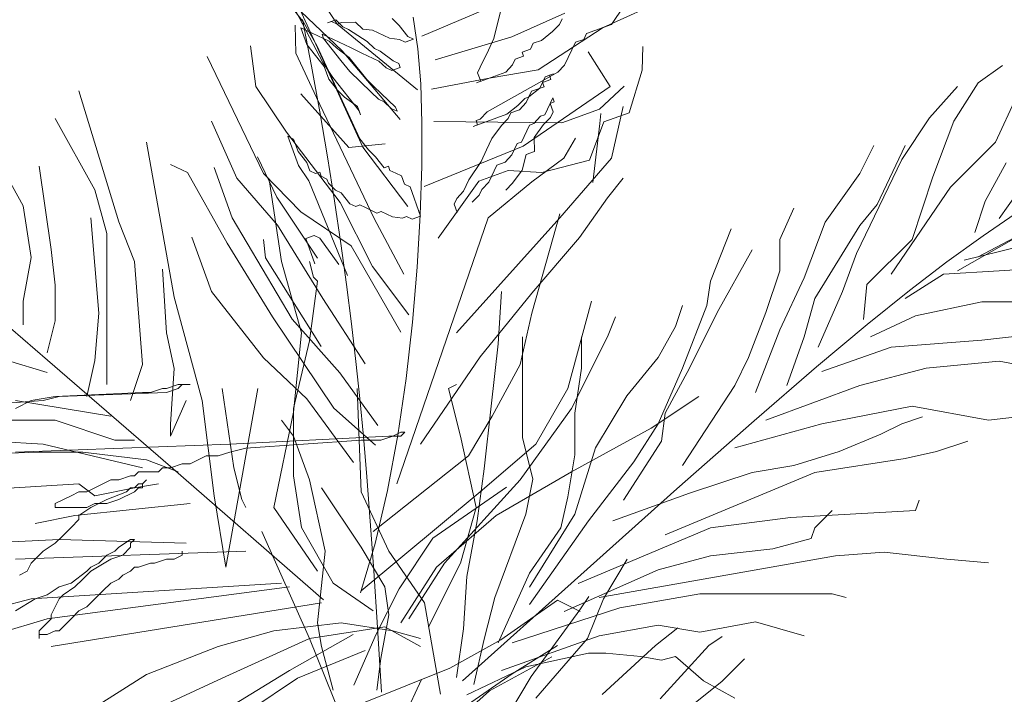
# Model space of a CAD drawing. Units: millimetres. Extents: x 595116 to 630915, y 909473 to 920225.
# Tile 37 of 134: x 629665.643 to 629671.98, y 919173.119 to 919177.461. Entities that reach past the tile are written whole.
import ezdxf

# ---------------------------------------------------------------- set-up
doc = ezdxf.new("R2010")
doc.units = ezdxf.units.MM
doc.layers.add('Dimension', color=3, linetype='Continuous', lineweight=18)
doc.layers.add('L-PLNT', color=85, linetype='Continuous', lineweight=13)
doc.styles.get("Standard").update_dxf_attribs({"font": 'arial.ttf'})
doc.dimstyles.new('ISO-25', dxfattribs={"dimtxt": 9, "dimasz": 6, "dimexe": 1.25, "dimexo": 0.625, "dimtad": 1, "dimlunit": 4, "dimtxsty": 'Standard', "dimcen": 2.5, "dimadec": 0, "dimazin": 0, "dimtfac": 1, "dimtmove": 0, "dimatfit": 3, "dimfxl": 1, "dimarcsym": 0})

# ---------------------------------------------------------------- blocks, each defined once
blk = doc.blocks.new('A$C4FB75ABC')
for p, q in [((2.6801, 3.4593), (2.5376, 3.6754)), ((2.6552, 3.3935), (2.5769, 3.5437)), ((3.136, 3.4531), (3.303, 3.5294)), ((2.6885, 3.4136), (2.5774, 3.5196)), ((2.5924, 3.5006), (2.6222, 3.4627)), ((2.7237, 3.248), (2.6067, 3.5058)), ((2.8253, 3.4385), (2.9518, 3.4922)), ((2.9484, 3.4342), (2.9616, 3.4876)), ((2.9797, 3.4374), (3.0703, 3.4781)), ((3.1503, 3.4583), (3.1713, 3.4901)), ((2.636, 3.3873), (2.6204, 3.467)), ((2.6222, 3.4627), (2.6449, 3.4222)), ((2.6632, 3.4613), (2.6776, 3.4664)), ((2.6704, 3.4639), (2.6632, 3.4613)), ((2.6801, 3.4593), (2.6704, 3.4639)), ((2.6776, 3.4664), (2.6899, 3.4547)), ((2.6873, 3.4618), (2.6801, 3.4593)), ((2.7114, 3.4624), (2.6873, 3.4618)), ((2.7237, 3.4506), (2.7114, 3.4624)), ((2.774, 3.4687), (2.7863, 3.4569)), ((2.81, 3.4712), (2.8183, 3.4166)), ((3.0657, 3.4683), (3.0611, 3.4586)), ((2.609, 3.4093), (2.6078, 3.4576)), ((2.6566, 3.4346), (2.6176, 3.453)), ((2.6176, 3.453), (2.6279, 3.4243)), ((2.8178, 3.3467), (2.6801, 3.4593)), ((2.6899, 3.4547), (2.6996, 3.4501)), ((2.6996, 3.4501), (2.7315, 3.4291)), ((2.7407, 3.4486), (2.7237, 3.4506)), ((2.7699, 3.4348), (2.7407, 3.4486)), ((2.7863, 3.4569), (2.8012, 3.438)), ((3.0244, 3.3805), (3.136, 3.4531)), ((3.0494, 3.4462), (3.0304, 3.4313)), ((3.0611, 3.4586), (3.0494, 3.4462)), ((3.1073, 3.4428), (3.1503, 3.4583)), ((2.6638, 3.4372), (2.654, 3.4418)), ((2.654, 3.4418), (2.6566, 3.4346)), ((2.6566, 3.4346), (2.6664, 3.43)), ((2.6865, 3.3967), (2.6566, 3.4346)), ((2.693, 3.4234), (2.6638, 3.4372)), ((2.6664, 3.43), (2.6787, 3.4182)), ((2.7315, 3.4291), (2.7438, 3.4173)), ((2.7869, 3.4328), (2.7699, 3.4348)), ((2.7966, 3.4282), (2.7869, 3.4328)), ((2.811, 3.4334), (2.7966, 3.4282)), ((2.8012, 3.438), (2.811, 3.4334)), ((2.848, 3.3981), (2.9797, 3.4374)), ((2.9392, 3.4147), (2.9484, 3.4342)), ((3.0304, 3.4313), (3.0161, 3.4262)), ((3.07, 3.3888), (3.0884, 3.4279)), ((3.0884, 3.4279), (3.1027, 3.433)), ((3.1027, 3.433), (3.1073, 3.4428)), ((2.5404, 3.3522), (2.5315, 3.422)), ((2.6279, 3.4243), (2.6578, 3.3864)), ((2.6449, 3.4222), (2.7186, 3.2624)), ((2.6787, 3.4182), (2.7008, 3.4019)), ((2.7877, 3.2953), (2.6885, 3.4136)), ((2.7028, 3.4188), (2.693, 3.4234)), ((2.7223, 3.4096), (2.7028, 3.4188)), ((2.7438, 3.4173), (2.7536, 3.4127)), ((2.7536, 3.4127), (2.7757, 3.3964)), ((2.8183, 3.4166), (2.8233, 3.3565)), ((2.9254, 3.3854), (2.9392, 3.4147)), ((3.0115, 3.4164), (2.9972, 3.4112)), ((2.9972, 3.4112), (2.9997, 3.4041)), ((3.0161, 3.4262), (3.0115, 3.4164)), ((3.1481, 3.3521), (3.1105, 3.4115)), ((3.2028, 3.3799), (3.2043, 3.4209)), ((2.5536, 3.203), (2.4572, 3.4034)), ((2.6446, 3.333), (2.609, 3.4093)), ((2.6727, 3.3674), (2.6552, 3.3935)), ((2.7014, 3.3777), (2.6865, 3.3967)), ((2.7008, 3.4019), (2.7306, 3.364)), ((2.7516, 3.3958), (2.7223, 3.4096)), ((2.7639, 3.384), (2.7516, 3.3958)), ((2.7757, 3.3964), (2.7854, 3.3918)), ((2.9854, 3.3989), (2.9808, 3.3891)), ((2.9997, 3.4041), (2.9854, 3.3989)), ((2.6503, 3.3086), (2.636, 3.3873)), ((2.6578, 3.3864), (2.6655, 3.3648)), ((2.7384, 3.3424), (2.7014, 3.3777)), ((2.7737, 3.3794), (2.7639, 3.384)), ((2.788, 3.3846), (2.7737, 3.3794)), ((2.7854, 3.3918), (2.788, 3.3846)), ((2.969, 3.3768), (2.9188, 3.3587)), ((2.9208, 3.3757), (2.9254, 3.3854)), ((2.9369, 3.3085), (3.0583, 3.3765)), ((2.9403, 3.3665), (3.0244, 3.3805)), ((2.9808, 3.3891), (2.969, 3.3768)), ((3.0583, 3.3765), (3.07, 3.3888)), ((3.1805, 3.307), (3.2028, 3.3799)), ((3.7791, 3.3582), (3.8208, 3.388)), ((2.6655, 3.3648), (2.6804, 3.3459)), ((2.7174, 3.3106), (2.6727, 3.3674)), ((2.7306, 3.364), (2.743, 3.3522)), ((2.8419, 3.3473), (2.9403, 3.3665)), ((2.9188, 3.3587), (2.926, 3.3613)), ((2.926, 3.3613), (2.9208, 3.3757)), ((3.0367, 3.3687), (3.0322, 3.359)), ((3.0322, 3.359), (3.0465, 3.3642)), ((3.0511, 3.3739), (3.0367, 3.3687)), ((3.0439, 3.3713), (3.0511, 3.3739)), ((3.0465, 3.3642), (3.0439, 3.3713)), ((2.2372, 3.345), (2.3054, 3.1203)), ((2.5929, 3.2739), (2.5404, 3.3522)), ((2.6804, 3.3459), (2.6928, 3.3341)), ((2.743, 3.3522), (2.7553, 3.3404)), ((2.8233, 3.3565), (2.8254, 3.2898)), ((2.9986, 3.2497), (3.1481, 3.3521)), ((3.0276, 3.3492), (3.0086, 3.3343)), ((3.0086, 3.3343), (3.0132, 3.3441)), ((3.0132, 3.3441), (3.0347, 3.3518)), ((3.0322, 3.359), (3.0276, 3.3492)), ((3.0347, 3.3518), (3.0322, 3.359)), ((3.1297, 3.313), (3.1722, 3.3526)), ((3.6956, 3.2986), (3.7433, 3.3522)), ((3.7373, 3.2926), (3.7791, 3.3582)), ((2.6997, 3.2474), (2.6179, 3.3396)), ((2.7435, 3.1255), (2.6446, 3.333)), ((2.6928, 3.3341), (2.7149, 3.3178)), ((2.7507, 3.3307), (2.7384, 3.3424)), ((2.7605, 3.3261), (2.7507, 3.3307)), ((2.7553, 3.3404), (2.78, 3.3169)), ((2.7728, 3.3143), (2.7605, 3.3261)), ((3.0015, 3.3317), (2.9897, 3.3194)), ((3.0086, 3.3343), (3.0015, 3.3317)), ((3.004, 3.3246), (3.0086, 3.3343)), ((3.0497, 3.3329), (3.0451, 3.3231)), ((3.0522, 3.3257), (3.0497, 3.3329)), ((3.8089, 3.2568), (3.8447, 3.3343)), ((2.7149, 3.3178), (2.72, 3.3034)), ((2.72, 3.3034), (2.7174, 3.3106)), ((2.7826, 3.3097), (2.7728, 3.3143)), ((2.78, 3.3169), (2.7826, 3.3097)), ((2.9897, 3.3194), (2.9708, 3.3045)), ((2.9779, 3.3071), (2.9923, 3.3122)), ((2.9923, 3.3122), (3.004, 3.3246)), ((3.0359, 3.3036), (3.0405, 3.3134)), ((3.0405, 3.3134), (3.0451, 3.3231)), ((3.0451, 3.3231), (3.0522, 3.3257)), ((3.0451, 3.3231), (3.0502, 3.3088)), ((3.0651, 3.2898), (3.1297, 3.313)), ((3.1501, 3.2292), (3.1706, 3.3178)), ((2.1963, 3.2973), (2.2645, 3.1748)), ((2.508, 3.1947), (2.4647, 3.2926)), ((2.6635, 3.2315), (2.6503, 3.3086)), ((2.9708, 3.3045), (2.9134, 3.2838)), ((2.918, 3.2936), (2.9251, 3.2962)), ((2.9206, 3.2864), (2.918, 3.2936)), ((2.9251, 3.2962), (2.9369, 3.3085)), ((2.9616, 3.285), (2.9733, 3.2973)), ((2.9733, 3.2973), (2.9779, 3.3071)), ((3.0169, 3.2887), (3.0287, 3.301)), ((3.0287, 3.301), (3.0359, 3.3036)), ((3.0456, 3.299), (3.0339, 3.2867)), ((3.0502, 3.3088), (3.0456, 3.299)), ((3.1303, 3.2889), (3.1323, 3.3059)), ((3.1374, 3.2915), (3.1805, 3.307)), ((3.6479, 3.227), (3.6956, 3.2986)), ((3.7015, 3.1972), (3.7373, 3.2926)), ((2.8254, 3.2898), (2.825, 3.2153)), ((2.8457, 3.2919), (3.0651, 3.2898)), ((2.9134, 3.2838), (2.9206, 3.2864)), ((2.9452, 3.2629), (2.9616, 3.285)), ((2.996, 3.2568), (3.0052, 3.2763)), ((3.0052, 3.2763), (3.0098, 3.2861)), ((3.0098, 3.2861), (3.0169, 3.2887)), ((3.0339, 3.2867), (3.0175, 3.2646)), ((3.1125, 3.2258), (3.1374, 3.2915)), ((3.1182, 3.1873), (3.1303, 3.2889)), ((2.685, 3.153), (2.5929, 3.2739)), ((2.6053, 3.2621), (2.5955, 3.2667)), ((2.5955, 3.2667), (2.6136, 3.2165)), ((2.613, 3.2406), (2.6053, 3.2621)), ((2.7186, 3.2624), (2.7335, 3.2434)), ((2.936, 3.2434), (2.9452, 3.2629)), ((3.0175, 3.2646), (3.0181, 3.2405)), ((3.0684, 3.2292), (3.0888, 3.2633)), ((2.353, 3.2565), (2.4007, 2.9909)), ((2.7622, 3.2537), (2.6997, 3.2474)), ((2.8009, 3.1461), (2.7237, 3.248)), ((2.7335, 3.2434), (2.7458, 3.2316)), ((2.829, 3.1805), (2.9986, 3.2497)), ((2.9269, 3.2238), (2.936, 3.2434)), ((2.9797, 3.2347), (2.9842, 3.2445)), ((2.9842, 3.2445), (2.9888, 3.2542)), ((2.9888, 3.2542), (2.996, 3.2568)), ((3.5763, 3.2032), (3.6001, 3.2509)), ((3.6061, 3.1495), (3.6538, 3.2509)), ((3.7314, 3.1793), (3.8089, 3.2568)), ((2.5763, 3.1625), (2.5433, 3.2317)), ((2.6279, 3.2216), (2.613, 3.2406)), ((2.6754, 3.1561), (2.6635, 3.2315)), ((2.7458, 3.2316), (2.7608, 3.2127)), ((2.9679, 3.2224), (2.9797, 3.2347)), ((3.0038, 3.2353), (2.9972, 3.2086)), ((3.0181, 3.2405), (3.0038, 3.2353)), ((3.0139, 3.1884), (3.0684, 3.2292)), ((3.031, 3.2046), (3.1125, 3.2258)), ((3.0616, 3.1271), (3.1501, 3.2292)), ((3.5703, 3.066), (3.6479, 3.227)), ((3.8149, 3.1257), (3.8865, 3.227)), ((2.1078, 3.2088), (2.1418, 3.1475)), ((2.1691, 3.2156), (2.1895, 3.0726)), ((2.4234, 3.2048), (2.3941, 3.2186)), ((2.5, 3.127), (2.469, 3.2131)), ((2.6136, 3.2165), (2.6311, 3.1904)), ((2.6331, 3.2073), (2.6279, 3.2216)), ((2.7608, 3.2127), (2.7679, 3.2153)), ((2.7679, 3.2153), (2.7705, 3.2081)), ((2.7705, 3.2081), (2.7803, 3.2035)), ((2.825, 3.2153), (2.8223, 3.1323)), ((2.9059, 3.192), (2.9269, 3.2238)), ((2.9229, 3.19), (2.9731, 3.208)), ((2.949, 3.2075), (2.9535, 3.2172)), ((2.9535, 3.2172), (2.9679, 3.2224)), ((2.9731, 3.208), (3.031, 3.2046)), ((2.9972, 3.2086), (2.9808, 3.1865)), ((3.791, 3.1555), (3.8268, 3.2211)), ((2.4914, 3.0833), (2.4234, 3.2048)), ((2.5774, 3.1143), (2.508, 3.1947)), ((2.6179, 3.137), (2.5536, 3.203)), ((2.6428, 3.2027), (2.6331, 3.2073)), ((2.65, 3.2053), (2.6428, 3.2027)), ((2.6526, 3.1981), (2.65, 3.2053)), ((2.6624, 3.1935), (2.6526, 3.1981)), ((2.6649, 3.1863), (2.6624, 3.1935)), ((2.7803, 3.2035), (2.79, 3.1989)), ((2.79, 3.1989), (2.7952, 3.1846)), ((2.8967, 3.1725), (2.9059, 3.192)), ((2.9398, 3.188), (2.949, 3.2075)), ((3.1433, 3.1611), (3.1706, 3.1952)), ((3.5166, 3.1197), (3.5763, 3.2032)), ((3.6658, 3.0899), (3.7015, 3.1972)), ((2.2645, 3.1748), (2.2849, 3.0999)), ((2.5847, 3.0522), (2.5642, 3.1884)), ((2.6311, 3.1904), (2.6976, 3.0279)), ((2.6773, 3.1746), (2.6649, 3.1863)), ((2.687, 3.17), (2.6773, 3.1746)), ((2.7952, 3.1846), (2.8049, 3.18)), ((2.8049, 3.18), (2.823, 3.1297)), ((2.8529, 3.0918), (2.9229, 3.19)), ((2.9234, 3.1659), (2.928, 3.1756)), ((2.928, 3.1756), (2.9398, 3.188)), ((2.9389, 3.1271), (3.0139, 3.1884)), ((2.9808, 3.1865), (2.969, 3.1742)), ((3.63, 3.0303), (3.7314, 3.1793)), ((2.6463, 3.058), (2.5763, 3.1625)), ((2.7019, 3.151), (2.687, 3.17)), ((2.8804, 3.1504), (2.885, 3.1601)), ((2.885, 3.1601), (2.8967, 3.1725)), ((2.9117, 3.1535), (2.9234, 3.1659)), ((3.0956, 3.093), (3.1433, 3.1611)), ((2.1418, 3.1475), (2.1555, 3.059)), ((2.6863, 3.0831), (2.6754, 3.1561)), ((2.7407, 3.0434), (2.685, 3.153)), ((2.7117, 3.1464), (2.7019, 3.151)), ((2.7189, 3.149), (2.7117, 3.1464)), ((2.7286, 3.1444), (2.7189, 3.149)), ((2.7481, 3.1352), (2.7286, 3.1444)), ((2.8856, 3.136), (2.8804, 3.1504)), ((3.4391, 3.0899), (3.4629, 3.1436)), ((3.5763, 3.1137), (3.6061, 3.1495)), ((3.7731, 3.1018), (3.791, 3.1555)), ((2.2577, 3.1271), (2.2713, 2.9637)), ((2.603, 2.9533), (2.5, 3.127)), ((2.7037, 3.0787), (2.6179, 3.137)), ((2.794, 3.0302), (2.7435, 3.1255)), ((2.7553, 3.1378), (2.7481, 3.1352)), ((2.7651, 3.1332), (2.7553, 3.1378)), ((2.7748, 3.1286), (2.7651, 3.1332)), ((2.7917, 3.1266), (2.7748, 3.1286)), ((2.7823, 2.6709), (2.9389, 3.1271)), ((2.7989, 3.1292), (2.7917, 3.1266)), ((2.8087, 3.1246), (2.7989, 3.1292)), ((2.823, 3.1297), (2.8087, 3.1246)), ((2.8223, 3.1323), (2.817, 3.0425)), ((2.8844, 2.9296), (3.0616, 3.1271)), ((3.0139, 2.9637), (3.0616, 3.1339)), ((3.7873, 3.0958), (3.8516, 3.1401)), ((2.3054, 3.1203), (2.3326, 3.0522)), ((2.6552, 2.9883), (2.5774, 3.1143)), ((3.3198, 3.0184), (3.3556, 3.1078)), ((3.4808, 3.0243), (3.5166, 3.1197)), ((3.4987, 2.9885), (3.5763, 3.1137)), ((3.7433, 3.0362), (3.8805, 3.1137)), ((3.7791, 3.0601), (3.8805, 3.1137)), ((2.2849, 3.0999), (2.2849, 2.9024)), ((2.4644, 3.0007), (2.4308, 3.094)), ((2.5571, 3.0584), (2.5539, 3.0896)), ((2.6406, 3.0965), (2.6262, 3.0913)), ((2.6262, 3.0913), (2.6417, 3.0483)), ((2.6503, 3.0919), (2.6406, 3.0965)), ((2.6827, 3.0468), (2.6503, 3.0919)), ((3.0139, 2.9977), (3.0956, 3.093)), ((3.4391, 3.0362), (3.4391, 3.0899)), ((3.5882, 3.0124), (3.6658, 3.0899)), ((3.7254, 3.0513), (3.7873, 3.0958)), ((2.1895, 3.0726), (2.1963, 3.0113)), ((2.5691, 2.9573), (2.4914, 3.0833)), ((2.696, 3.0126), (2.6863, 3.0831)), ((2.7892, 2.9311), (2.7037, 3.0787)), ((3.7552, 3.0541), (3.8507, 3.078)), ((2.1555, 3.059), (2.1418, 2.9841)), ((2.6523, 2.9062), (2.5571, 3.0584)), ((3.3317, 2.9647), (3.3914, 3.072)), ((3.5465, 3.0005), (3.5703, 3.066)), ((2.3326, 3.0522), (2.3462, 2.8751)), ((2.6187, 2.9296), (2.5847, 3.0522)), ((2.6392, 3.0249), (2.6324, 3.0522)), ((2.8029, 2.9604), (2.7407, 3.0434)), ((2.817, 3.0425), (2.809, 2.948)), ((3.6611, 3.0024), (3.7254, 3.0513)), ((3.8149, 3.0362), (3.9222, 3.0422)), ((2.1835, 2.8826), (2.0174, 3.0255)), ((2.3803, 3.0386), (2.3871, 2.9296)), ((2.646, 3.0181), (2.6392, 3.0249)), ((3.4152, 2.9647), (3.4391, 3.0362)), ((3.4391, 2.9349), (3.4808, 3.0243)), ((3.6538, 2.9885), (3.7194, 3.0303)), ((3.7194, 3.0303), (3.8149, 3.0362)), ((2.1963, 3.0113), (2.1963, 2.95)), ((2.6324, 2.916), (2.646, 3.0181)), ((2.7046, 2.9452), (2.696, 3.0126)), ((3.3138, 2.9766), (3.3198, 3.0184)), ((3.5822, 2.9528), (3.5882, 3.0124)), ((2.4007, 2.9909), (2.4484, 2.8139)), ((2.5539, 2.887), (2.4644, 3.0007)), ((2.7278, 2.8766), (2.6552, 2.9883)), ((2.9253, 2.8888), (3.0139, 2.9977)), ((2.9559, 2.911), (2.9619, 3.0005)), ((3.4808, 2.923), (3.4987, 2.9885)), ((3.5047, 2.9051), (3.5465, 3.0005)), ((3.5886, 2.9442), (3.6611, 3.0024)), ((2.1418, 2.9841), (2.1418, 2.9432)), ((3.0752, 2.8343), (3.1161, 2.9841)), ((3.2601, 2.9408), (3.2721, 2.9766)), ((3.2721, 2.8693), (3.3138, 2.9766)), ((3.6717, 2.9587), (3.7851, 2.9826)), ((3.7851, 2.9826), (3.8745, 2.9826)), ((2.2713, 2.9637), (2.2645, 2.882)), ((2.6741, 2.8006), (2.5691, 2.9573)), ((2.9935, 2.8751), (3.0139, 2.9637)), ((3.1433, 2.9228), (3.157, 2.9569)), ((3.284, 2.8693), (3.3317, 2.9647)), ((3.3854, 2.8872), (3.4152, 2.9647)), ((3.5942, 2.923), (3.6717, 2.9587)), ((2.1963, 2.95), (2.1827, 2.8956)), ((2.6847, 2.8611), (2.603, 2.9533)), ((2.7122, 2.8807), (2.7046, 2.9452)), ((2.809, 2.948), (2.7981, 2.8512)), ((3.2303, 2.8872), (3.2601, 2.9408)), ((3.5019, 2.8714), (3.5886, 2.9442)), ((2.3871, 2.9296), (2.4007, 2.8683)), ((2.6051, 2.7934), (2.6187, 2.9296)), ((2.9977, 2.8216), (2.9977, 2.923)), ((3.082, 2.8002), (3.1433, 2.9228)), ((3.0991, 2.8693), (3.0991, 2.923)), ((3.3973, 2.8276), (3.4391, 2.9349)), ((3.451, 2.8395), (3.4808, 2.923)), ((3.7851, 2.917), (3.8924, 2.9289)), ((2.6051, 2.8002), (2.6324, 2.916)), ((2.944, 2.8037), (2.9559, 2.911)), ((3.5107, 2.8633), (3.63, 2.9051)), ((3.63, 2.9051), (3.7851, 2.917)), ((2.2849, 2.9024), (2.2849, 2.8411)), ((2.6279, 2.8164), (2.5539, 2.887)), ((2.8231, 2.739), (2.9253, 2.8888)), ((3.1766, 2.8216), (3.2303, 2.8872)), ((3.3615, 2.8395), (3.3854, 2.8872)), ((2.1146, 2.882), (2.1827, 2.8615)), ((2.3943, 2.7002), (2.1835, 2.8826)), ((2.2645, 2.882), (2.2508, 2.8207)), ((2.3462, 2.8751), (2.3258, 2.8139)), ((2.7189, 2.8171), (2.7122, 2.8807)), ((2.9458, 2.7866), (2.9935, 2.8751)), ((3.3951, 2.779), (3.5019, 2.8714)), ((3.6896, 2.8693), (3.8149, 2.8812)), ((3.8149, 2.8812), (3.9103, 2.8633)), ((2.4007, 2.8683), (2.3939, 2.773)), ((2.7496, 2.771), (2.6847, 2.8611)), ((3.0872, 2.7918), (3.0991, 2.8693)), ((3.2303, 2.7739), (3.2721, 2.8693)), ((3.2422, 2.7918), (3.284, 2.8693)), ((3.5763, 2.8395), (3.6896, 2.8693)), ((2.3871, 2.8343), (2.4075, 2.8411)), ((2.4075, 2.8411), (2.428, 2.8411)), ((2.4144, 2.8411), (2.4075, 2.8343)), ((2.428, 2.8411), (2.4144, 2.8411)), ((2.7981, 2.8512), (2.784, 2.7542)), ((2.8708, 2.8343), (2.8844, 2.8411)), ((3.2721, 2.7024), (3.3615, 2.8395)), ((3.4152, 2.7799), (3.5763, 2.8395)), ((2.1555, 2.8139), (2.1963, 2.8207)), ((2.2032, 2.8207), (2.1759, 2.8139)), ((2.1963, 2.8207), (2.3462, 2.8275)), ((2.3871, 2.8275), (2.2032, 2.8207)), ((2.3462, 2.8275), (2.3599, 2.8275)), ((2.3599, 2.8275), (2.3803, 2.8343)), ((2.3803, 2.8343), (2.3871, 2.8343)), ((2.4075, 2.8343), (2.3871, 2.8275)), ((2.4825, 2.8343), (2.5029, 2.6981)), ((2.4893, 2.5279), (2.5438, 2.8343)), ((2.7209, 2.6572), (2.7141, 2.8343)), ((2.8913, 2.7526), (2.8708, 2.8343)), ((2.9977, 2.7501), (2.9977, 2.8216)), ((3.0207, 2.739), (3.0752, 2.8343)), ((3.1229, 2.7322), (3.1766, 2.8216)), ((3.2183, 2.7662), (3.3, 2.8207)), ((2.1759, 2.8139), (2.0056, 2.8002)), ((2.1282, 2.8002), (2.1555, 2.8139)), ((2.1282, 2.8139), (2.2917, 2.7866)), ((2.3939, 2.7526), (2.4212, 2.8139)), ((2.4484, 2.8139), (2.4689, 2.6504)), ((2.7077, 2.7073), (2.6279, 2.8164)), ((2.7251, 2.7519), (2.7189, 2.8171)), ((2.9321, 2.6964), (2.944, 2.8037)), ((3.5107, 2.7739), (3.6658, 2.8037)), ((3.6658, 2.8037), (3.797, 2.7799)), ((2.5711, 2.63), (2.6051, 2.7934)), ((2.6051, 2.6845), (2.6051, 2.8002)), ((2.7456, 2.7371), (2.6741, 2.8006)), ((2.9049, 2.7185), (2.9458, 2.7866)), ((2.9935, 2.6777), (3.082, 2.8002)), ((3.0872, 2.7203), (3.0872, 2.7918)), ((3.2363, 2.7441), (3.2422, 2.7918)), ((3.6479, 2.7739), (3.6837, 2.7858)), ((3.797, 2.7799), (3.8984, 2.7918)), ((2.1078, 2.7798), (2.1963, 2.7798)), ((2.1963, 2.7798), (2.2985, 2.7458)), ((2.3939, 2.773), (2.3939, 2.7526)), ((2.6051, 2.7526), (2.5847, 2.7798)), ((3.1886, 2.7083), (3.2303, 2.7739)), ((3.2623, 2.6619), (3.3951, 2.779)), ((3.3615, 2.7322), (3.5107, 2.7739)), ((3.6121, 2.756), (3.6479, 2.7739)), ((2.4961, 2.739), (2.7686, 2.7526)), ((2.6324, 2.6777), (2.6051, 2.7526)), ((2.7309, 2.6826), (2.7251, 2.7519)), ((2.7754, 2.7526), (2.755, 2.7458)), ((2.784, 2.7542), (2.7664, 2.6591)), ((2.7686, 2.7526), (2.7891, 2.7526)), ((2.7891, 2.7594), (2.7754, 2.7526)), ((2.7891, 2.7526), (2.7959, 2.7594)), ((2.7959, 2.7594), (2.7891, 2.7594)), ((2.9185, 2.63), (2.8913, 2.7526)), ((3.082, 2.6913), (3.2183, 2.7662)), ((3.5405, 2.7262), (3.6121, 2.756)), ((2.1759, 2.739), (2.0601, 2.7458)), ((2.3462, 2.6981), (2.1759, 2.739)), ((2.2985, 2.7458), (2.3326, 2.7458)), ((2.3122, 2.7321), (2.4961, 2.739)), ((2.7209, 2.7458), (2.5234, 2.7321)), ((2.755, 2.7458), (2.7209, 2.7458)), ((2.9253, 2.6572), (3.0207, 2.739)), ((3.0156, 2.6785), (2.9977, 2.7501)), ((3.1707, 2.6428), (3.2363, 2.7441)), ((3.7075, 2.7262), (3.7612, 2.7441)), ((1.8285, 2.7117), (2.1691, 2.7253)), ((2.1282, 2.7253), (2.3122, 2.7321)), ((2.1691, 2.7253), (2.244, 2.7253)), ((2.244, 2.7253), (2.353, 2.7117)), ((2.4552, 2.7185), (2.428, 2.7049)), ((2.4757, 2.7185), (2.4552, 2.7185)), ((2.4961, 2.7253), (2.4757, 2.7185)), ((2.5234, 2.7321), (2.4961, 2.7253)), ((2.7414, 2.5891), (2.9049, 2.7185)), ((3.0752, 2.6487), (3.0872, 2.7203)), ((3.0872, 2.6189), (3.1229, 2.7322)), ((3.4629, 2.7024), (3.5405, 2.7262)), ((3.6538, 2.7143), (3.7075, 2.7262)), ((2.353, 2.7117), (2.4075, 2.6913)), ((2.4144, 2.7049), (2.3939, 2.6981)), ((2.428, 2.7049), (2.4144, 2.7049)), ((3.111, 2.607), (3.1886, 2.7083)), ((3.3914, 2.6904), (3.4629, 2.7024)), ((3.4987, 2.6904), (3.6538, 2.7143)), ((2.3258, 2.6845), (2.3054, 2.6777)), ((2.3326, 2.6845), (2.3258, 2.6845)), ((2.3394, 2.6913), (2.3326, 2.6845)), ((2.3735, 2.6913), (2.3394, 2.6913)), ((2.3803, 2.6981), (2.3735, 2.6913)), ((2.3939, 2.6981), (2.3803, 2.6981)), ((2.6566, 2.472), (2.3943, 2.7002)), ((2.5029, 2.6981), (2.5166, 2.6436)), ((2.6187, 2.596), (2.6051, 2.6845)), ((2.9201, 2.607), (2.9321, 2.6964)), ((2.9526, 2.6164), (3.082, 2.6913)), ((3.2422, 2.5831), (3.4987, 2.6904)), ((3.284, 2.6547), (3.3914, 2.6904)), ((1.917, 2.6504), (2.2372, 2.6709)), ((2.2372, 2.6709), (2.2645, 2.6504)), ((2.2917, 2.6777), (2.2508, 2.6572)), ((2.3054, 2.6777), (2.2917, 2.6777)), ((2.3394, 2.6709), (2.3326, 2.664)), ((2.3326, 2.664), (2.3735, 2.6709)), ((2.3462, 2.6709), (2.3394, 2.6709)), ((2.3462, 2.6709), (2.353, 2.6777)), ((2.353, 2.6777), (2.3462, 2.6709)), ((2.3462, 2.664), (2.3462, 2.6709)), ((2.6596, 2.5551), (2.6324, 2.6777)), ((2.7367, 2.6065), (2.7309, 2.6826)), ((2.864, 2.5347), (2.9935, 2.6777)), ((3.0036, 2.6189), (3.0156, 2.6785)), ((2.2372, 2.6572), (2.2236, 2.6504)), ((2.2508, 2.6572), (2.2372, 2.6572)), ((2.2645, 2.6504), (2.3326, 2.664)), ((2.319, 2.6572), (2.2849, 2.6436)), ((2.3054, 2.6436), (2.3326, 2.6572)), ((2.3258, 2.664), (2.319, 2.6572)), ((2.3326, 2.664), (2.3258, 2.664)), ((2.3326, 2.6572), (2.3394, 2.664)), ((2.3394, 2.664), (2.3462, 2.664)), ((2.6528, 2.664), (2.7209, 2.5619)), ((2.7209, 2.487), (2.9253, 2.6572)), ((2.7686, 2.5551), (2.7209, 2.6572)), ((2.7664, 2.6591), (2.7451, 2.5683)), ((2.8442, 2.5778), (2.9704, 2.6651)), ((3.0976, 2.5149), (3.2623, 2.6619)), ((3.1528, 2.607), (3.284, 2.6547)), ((2.2236, 2.6504), (2.1963, 2.6368)), ((2.1963, 2.6368), (2.1963, 2.63)), ((2.428, 2.6368), (2.2304, 2.6164)), ((2.2508, 2.63), (2.2645, 2.6368)), ((2.2849, 2.6436), (2.2577, 2.63)), ((2.2645, 2.6368), (2.2849, 2.6368)), ((2.2849, 2.6368), (2.3054, 2.6436)), ((2.4689, 2.6504), (2.4893, 2.5279)), ((2.5166, 2.6436), (2.5234, 2.63)), ((3.0633, 2.5951), (3.0752, 2.6487)), ((3.6717, 2.6249), (3.6777, 2.6428)), ((2.1963, 2.63), (2.2508, 2.63)), ((2.2577, 2.63), (2.2372, 2.6164)), ((2.646, 2.5211), (2.5711, 2.63)), ((2.8913, 2.5347), (2.9185, 2.63)), ((2.95, 2.4758), (3.0036, 2.6189)), ((3.0096, 2.4937), (3.0872, 2.6189)), ((3.457, 2.6129), (3.6717, 2.6249)), ((3.4987, 2.5951), (3.5286, 2.6249)), ((2.2304, 2.6164), (2.1623, 2.6028)), ((2.2372, 2.6096), (2.2236, 2.596)), ((2.2372, 2.6164), (2.2372, 2.6096)), ((2.7426, 2.5213), (2.7367, 2.6065)), ((2.8504, 2.5279), (2.9526, 2.6164)), ((2.9022, 2.5116), (2.9201, 2.607)), ((3.0096, 2.4639), (3.111, 2.607)), ((3.3198, 2.5951), (3.457, 2.6129)), ((2.2236, 2.596), (2.21, 2.5823)), ((2.5506, 2.5891), (2.6324, 2.4053)), ((2.6732, 2.5006), (2.6187, 2.596)), ((3.0096, 2.5176), (3.0633, 2.5951)), ((3.0931, 2.4997), (3.3198, 2.5951)), ((3.4928, 2.5772), (3.4987, 2.5951)), ((2.2032, 2.5755), (2.0737, 2.5687)), ((2.1963, 2.5687), (2.1759, 2.5551)), ((2.21, 2.5823), (2.1963, 2.5687)), ((2.4212, 2.5687), (2.2032, 2.5755)), ((2.3054, 2.5619), (2.3258, 2.5755)), ((2.3258, 2.5755), (2.3326, 2.5755)), ((2.3326, 2.5755), (2.3258, 2.5687)), ((2.3258, 2.5687), (2.3258, 2.5619)), ((2.7451, 2.5683), (2.72, 2.484)), ((2.786, 2.4905), (2.8442, 2.5778)), ((3.4272, 2.5593), (3.4928, 2.5772)), ((2.5234, 2.5551), (2.1282, 2.5415)), ((2.1759, 2.5551), (2.1623, 2.5415)), ((2.2849, 2.5483), (2.2985, 2.5551)), ((2.2985, 2.5551), (2.3054, 2.5619)), ((2.3258, 2.5619), (2.3122, 2.5483)), ((2.4144, 2.5483), (2.4144, 2.5551)), ((2.646, 2.4325), (2.6596, 2.5551)), ((2.7209, 2.5619), (2.7618, 2.4938)), ((2.8299, 2.4666), (2.7686, 2.5551)), ((3.3198, 2.5474), (3.4272, 2.5593)), ((3.5345, 2.5474), (3.618, 2.5533)), ((3.618, 2.5533), (3.7254, 2.5414)), ((2.1555, 2.5347), (2.1487, 2.5211)), ((2.1623, 2.5415), (2.1555, 2.5347)), ((2.2917, 2.5415), (2.2577, 2.5211)), ((2.2577, 2.5279), (2.2713, 2.5347)), ((2.2713, 2.5347), (2.2781, 2.5415)), ((2.2781, 2.5415), (2.2849, 2.5483)), ((2.3122, 2.5483), (2.2917, 2.5415)), ((2.3394, 2.5279), (2.3599, 2.5347)), ((2.3599, 2.5347), (2.3667, 2.5347)), ((2.3667, 2.5347), (2.3871, 2.5415)), ((2.3871, 2.5415), (2.4007, 2.5415)), ((2.4007, 2.5415), (2.4144, 2.5483)), ((2.8027, 2.4393), (2.864, 2.5347)), ((2.8368, 2.4257), (2.8913, 2.5347)), ((3.1289, 2.4758), (3.5345, 2.5474)), ((3.1365, 2.4734), (3.1774, 2.5415)), ((3.2303, 2.5235), (3.3198, 2.5474)), ((3.7254, 2.5414), (3.797, 2.5354)), ((2.1487, 2.5211), (2.135, 2.5142)), ((2.2236, 2.5006), (2.2508, 2.5211)), ((2.2577, 2.5211), (2.244, 2.5074)), ((2.2508, 2.5211), (2.2577, 2.5279)), ((2.3122, 2.5142), (2.3258, 2.5211)), ((2.3258, 2.5211), (2.3326, 2.5279)), ((2.3326, 2.5279), (2.3394, 2.5279)), ((2.7489, 2.4244), (2.7426, 2.5213)), ((2.7891, 2.4325), (2.8504, 2.5279)), ((2.9559, 2.3983), (3.0096, 2.5176)), ((3.0693, 2.452), (3.2303, 2.5235)), ((2.5847, 2.5006), (2.1555, 2.4734)), ((2.2032, 2.4938), (2.2236, 2.5006)), ((2.244, 2.5074), (2.2304, 2.4938)), ((2.2781, 2.487), (2.2917, 2.5006)), ((2.2917, 2.5006), (2.3054, 2.5074)), ((2.3054, 2.5074), (2.3122, 2.5142)), ((2.7414, 2.453), (2.6732, 2.5006)), ((2.895, 2.333), (3.0976, 2.5149)), ((2.8963, 2.4222), (2.9022, 2.5116)), ((2.1827, 2.4802), (2.2032, 2.4938)), ((2.5983, 2.4938), (2.1827, 2.4393)), ((2.2304, 2.4938), (2.21, 2.4802)), ((2.2508, 2.4598), (2.2781, 2.487)), ((2.7471, 2.4129), (2.786, 2.4905)), ((2.7618, 2.4938), (2.7686, 2.4461)), ((3.1647, 2.4579), (3.3019, 2.4818)), ((3.3019, 2.4818), (3.4152, 2.4818)), ((3.4152, 2.4818), (3.5286, 2.4818)), ((3.5286, 2.4818), (3.5524, 2.4758)), ((2.1555, 2.4734), (2.026, 2.4393)), ((2.1282, 2.453), (2.1623, 2.4734)), ((2.1623, 2.4734), (2.1827, 2.4802)), ((2.6528, 2.4666), (2.1895, 2.3917)), ((2.2032, 2.4734), (2.1963, 2.4598)), ((2.21, 2.4802), (2.2032, 2.4734)), ((2.8572, 2.31), (2.8299, 2.4666)), ((2.9321, 2.4043), (2.95, 2.4758)), ((2.9607, 2.4032), (3.0578, 2.4711)), ((3.0578, 2.4711), (3.0966, 2.4517)), ((3.0962, 2.4544), (3.1115, 2.4773)), ((3.1093, 2.4053), (3.1365, 2.4734)), ((2.1963, 2.4598), (2.1895, 2.4461)), ((2.2236, 2.4393), (2.2372, 2.453)), ((2.2372, 2.453), (2.2508, 2.4598)), ((2.9798, 2.3983), (3.1647, 2.4579)), ((3.0123, 2.3401), (3.0962, 2.4544)), ((2.1827, 2.4393), (1.9579, 2.3712)), ((2.1895, 2.4393), (2.1759, 2.4257)), ((2.1895, 2.4461), (2.1895, 2.4393)), ((2.2032, 2.4189), (2.2236, 2.4393)), ((2.5711, 2.4189), (2.6869, 2.4325)), ((2.6528, 2.3917), (2.646, 2.4325)), ((2.6869, 2.4325), (2.7754, 2.4189)), ((2.7686, 2.4461), (2.755, 2.3712)), ((3.3019, 2.4162), (3.3973, 2.4341)), ((3.3973, 2.4341), (3.4808, 2.4102)), ((2.1759, 2.4257), (2.1691, 2.4189)), ((2.1691, 2.4189), (2.1691, 2.4053)), ((2.1827, 2.4121), (2.1963, 2.4189)), ((2.1963, 2.4189), (2.2032, 2.4189)), ((2.4757, 2.3917), (2.5711, 2.4189)), ((2.6324, 2.4053), (2.7618, 2.4257)), ((2.7559, 2.3132), (2.7489, 2.4244)), ((2.7618, 2.4257), (2.8231, 2.3917)), ((2.7754, 2.4189), (2.8231, 2.4053)), ((2.8844, 2.3387), (2.8963, 2.4222)), ((3.1289, 2.4102), (3.2303, 2.4281)), ((3.2259, 2.3934), (3.264, 2.4239)), ((3.2303, 2.4281), (3.3019, 2.4162)), ((2.1691, 2.4053), (2.1691, 2.4121)), ((2.1691, 2.4121), (2.1827, 2.4121)), ((2.4825, 2.3372), (2.6324, 2.4053)), ((2.7073, 2.4121), (2.5983, 2.3508)), ((2.6324, 2.4053), (2.7073, 2.2214)), ((2.7083, 2.3255), (2.7471, 2.4129)), ((2.8733, 2.3546), (2.9607, 2.4032)), ((2.9142, 2.3268), (2.9321, 2.4043)), ((2.9619, 2.3506), (3.1289, 2.4102)), ((3.0207, 2.3031), (3.1093, 2.4053)), ((3.3174, 2.3934), (3.3403, 2.4087)), ((2.353, 2.344), (2.4757, 2.3917)), ((2.7277, 2.3849), (2.6119, 2.3372)), ((2.6732, 2.3168), (2.6528, 2.3917)), ((2.9801, 2.3449), (3.0578, 2.3935)), ((3.0036, 2.3566), (3.111, 2.3804)), ((3.111, 2.3804), (3.1408, 2.3804)), ((3.1344, 2.3096), (3.2259, 2.3934)), ((3.1408, 2.3804), (3.2005, 2.3745)), ((3.2335, 2.302), (3.3174, 2.3934)), ((2.755, 2.3712), (2.7482, 2.3168)), ((2.9413, 2.3158), (3.0481, 2.3741)), ((3.2005, 2.3745), (3.2363, 2.3685)), ((3.2363, 2.3685), (3.2601, 2.3745)), ((3.2601, 2.3745), (3.3079, 2.3327)), ((3.3403, 2.3324), (3.3784, 2.3706)), ((2.5983, 2.3508), (2.4757, 2.2759)), ((2.7277, 2.2964), (2.8733, 2.3546)), ((2.9022, 2.3089), (3.0036, 2.3566)), ((2.2781, 2.2963), (2.353, 2.344)), ((2.3054, 2.2555), (2.4825, 2.3372)), ((2.6119, 2.3372), (2.5302, 2.2827)), ((2.8248, 2.3352), (2.7471, 2.1703)), ((2.8539, 2.2576), (2.9801, 2.3449)), ((2.9666, 2.2638), (3.0123, 2.3401)), ((3.264, 2.2715), (3.3403, 2.3324)), ((3.3079, 2.3327), (3.3615, 2.3029)), ((2.8539, 2.2382), (2.9413, 2.3158))]:
    blk.add_line(p, q)
blk = doc.blocks.new('*D216')
at = {"layer": 'Defpoints', "color": 0, "transparency": 16777216}
for p in [(629743.5408, 919411.9276), (629505.0408, 919411.8279), (629743.5408, 918832.3776)]:
    blk.add_point(p, dxfattribs=at)
at = {"layer": 'Dimension', "color": 0, "lineweight": -2, "transparency": 16777216}
for p, q in [((629743.5408, 919411.3026), (629743.5408, 918831.1276)), ((629505.0408, 919411.2029), (629505.0408, 918831.1276)), ((629511.0408, 918832.3776), (629737.5408, 918832.3776))]:
    blk.add_line(p, q, dxfattribs=at)
at = {"layer": 'Dimension', "color": 0, "transparency": 16777216}
for points in [[(629511.0408, 918833.3776), (629511.0408, 918831.3776), (629505.0408, 918832.3776)], [(629737.5408, 918833.3776), (629737.5408, 918831.3776), (629743.5408, 918832.3776)]]:
    blk.add_solid(points, dxfattribs=at)
at = {"layer": 'Dimension', "color": 0, "transparency": 16777216, "insert": (629624.2908, 918837.656), "char_height": 9, "attachment_point": 5}
blk.add_mtext('19\'-10 1/2"', dxfattribs=at)

msp = doc.modelspace()

# ---------------------------------------------------------------- block references
at = {"layer": 'L-PLNT', "xscale": 3.753413438031968, "yscale": 3.753413438031968, "zscale": 3.753413438031968}
msp.add_blockref('A$C4FB75ABC', (629657.6275, 919164.4492), dxfattribs=at)

# ---------------------------------------------------------------- dimensions: what is measured, and where the dimension line sits
at = {"layer": 'Dimension'}
dim = msp.add_linear_dim(base=(629743.5408, 918832.3776), p1=(629505.0408, 919411.8279), p2=(629743.5408, 919411.9276), dimstyle='ISO-25', override={"dimdec": 1, "dimlfac": 1, "dimrnd": 0, "dimzin": 1, "dimdsep": 46, "dimlunit": 4, "dimfrac": 2}, dxfattribs=at)
dim.commit()
dim.dimension.update_dxf_attribs({"geometry": '*D216', "text_midpoint": (629624.2908, 918837.656)})

doc.saveas('drawing.dxf')
